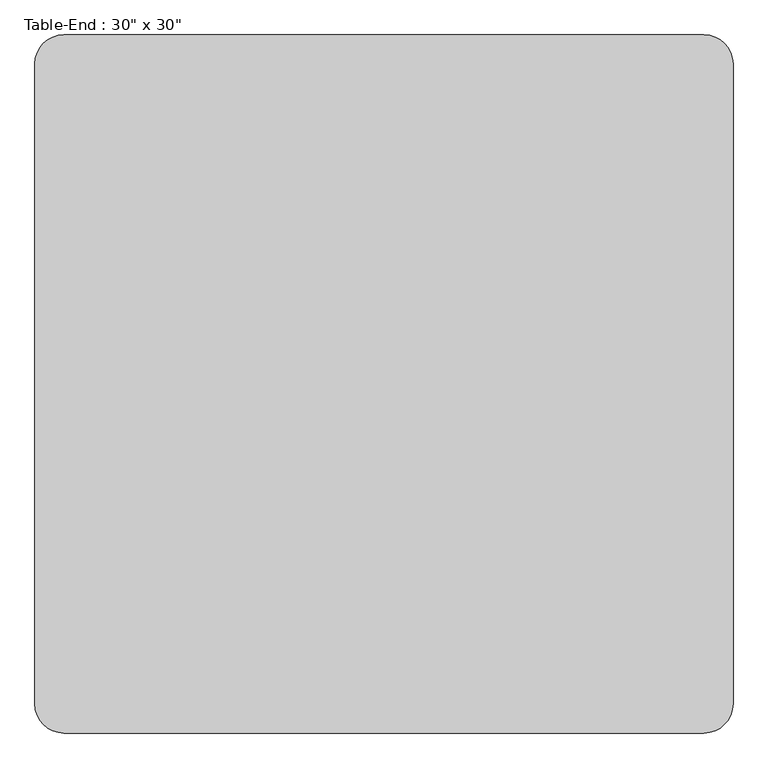
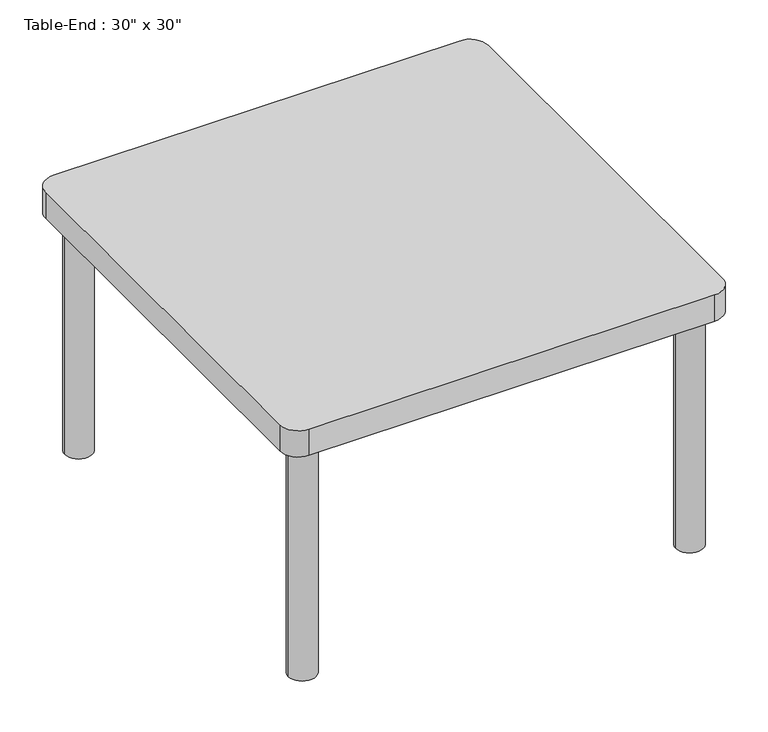
"""IFC4 building model written with IfcOpenShell, lengths in millimetres: furniture geometry."""

from ifc_helpers import new_model, si_unit, point, frame, frame_2d, origin, origin_with_axes, place, context, project, spatial, polyline, circle_curve, trimmed, segment, composite_curve, outline, extrude, source, transform, mapped, element, save


def furniture_e4e19c7b(model_context):
    return source(origin(), model_context, "Body", "SweptSolid", [
        extrude(outline(composite_curve([segment(polyline([(1172.1336303, -457.2), (54.5336303, -457.2)]), True, "CONTINUOUS"), segment(trimmed(circle_curve(frame_2d((54.5336303, -406.4)), 50.8), [point((54.5336303, -457.2))], [point((3.7336303, -406.4))], False, "CARTESIAN"), True, "CONTINUOUS"), segment(polyline([(3.7336303, -406.4), (3.7336303, 711.2)]), True, "CONTINUOUS"), segment(trimmed(circle_curve(frame_2d((54.5336303, 711.2)), 50.8), [point((3.7336303, 711.2))], [point((54.5336303, 762.0))], False, "CARTESIAN"), True, "CONTINUOUS"), segment(polyline([(54.5336303, 762.0), (1172.1336303, 762.0)]), True, "CONTINUOUS"), segment(trimmed(circle_curve(frame_2d((1172.1336303, 711.2)), 50.8), [point((1172.1336303, 762.0))], [point((1222.9336303, 711.2))], False, "CARTESIAN"), True, "CONTINUOUS"), segment(polyline([(1222.9336303, 711.2), (1222.9336303, -406.4)]), True, "CONTINUOUS"), segment(trimmed(circle_curve(frame_2d((1172.1336303, -406.4)), 50.8), [point((1222.9336303, -406.4))], [point((1172.1336303, -457.2))], False, "CARTESIAN"), True, "CONTINUOUS")], self_intersect=False)), frame((0.0, 0.0, 685.8), z_axis=(0.0, 0.0, 1.0), x_axis=(1.0, 0.0, 0.0)), (0.0, 0.0, 1.0), 76.2),
        extrude(outline(composite_curve([segment(trimmed(circle_curve(frame_2d((79.9336303, 685.8)), 38.1), [point((41.8336303, 685.8))], [point((118.0336303, 685.8))], False, "CARTESIAN"), True, "CONTINUOUS"), segment(trimmed(circle_curve(frame_2d((79.9336303, 685.8)), 38.1), [point((118.0336303, 685.8))], [point((41.8336303, 685.8))], False, "CARTESIAN"), True, "CONTINUOUS")], self_intersect=False)), origin_with_axes(), (0.0, 0.0, 1.0), 685.8),
        extrude(outline(composite_curve([segment(trimmed(circle_curve(frame_2d((79.9336303, -381.0)), 38.1), [point((41.8336303, -381.0))], [point((118.0336303, -381.0))], False, "CARTESIAN"), True, "CONTINUOUS"), segment(trimmed(circle_curve(frame_2d((79.9336303, -381.0)), 38.1), [point((118.0336303, -381.0))], [point((41.8336303, -381.0))], False, "CARTESIAN"), True, "CONTINUOUS")], self_intersect=False)), origin_with_axes(), (0.0, 0.0, 1.0), 685.8),
        extrude(outline(composite_curve([segment(trimmed(circle_curve(frame_2d((1146.7336303, -381.0)), 38.1), [point((1108.6336303, -381.0))], [point((1184.8336303, -381.0))], False, "CARTESIAN"), True, "CONTINUOUS"), segment(trimmed(circle_curve(frame_2d((1146.7336303, -381.0)), 38.1), [point((1184.8336303, -381.0))], [point((1108.6336303, -381.0))], False, "CARTESIAN"), True, "CONTINUOUS")], self_intersect=False)), origin_with_axes(), (0.0, 0.0, 1.0), 685.8),
        extrude(outline(composite_curve([segment(trimmed(circle_curve(frame_2d((1146.7336303, 685.8)), 38.1), [point((1108.6336303, 685.8))], [point((1184.8336303, 685.8))], False, "CARTESIAN"), True, "CONTINUOUS"), segment(trimmed(circle_curve(frame_2d((1146.7336303, 685.8)), 38.1), [point((1184.8336303, 685.8))], [point((1108.6336303, 685.8))], False, "CARTESIAN"), True, "CONTINUOUS")], self_intersect=False)), origin_with_axes(), (0.0, 0.0, 1.0), 685.8),
    ])


if __name__ == "__main__":
    model = new_model("IFC4")
    model_context = context("Model", 3, world=origin())
    ifc_project = project(units=[si_unit("LENGTHUNIT", "METRE", prefix="MILLI")], contexts=[model_context])
    site = spatial("IfcSite", under=ifc_project)
    building = spatial("IfcBuilding", under=site)
    placement = place(None, origin())
    furniture_shape = furniture_e4e19c7b(model_context)
    element("IfcFurniture", 1, ObjectType="Table-End : 30\" x 30\"", at=placement, inside=building, context=model_context, shape_type="MappedRepresentation", body=[
        mapped(furniture_shape, transform((0.0, 0.0, 0.0), x_axis=(1.0, 0.0, 0.0), y_axis=(0.0, 1.0, 0.0), z_axis=(0.0, 0.0, 1.0))),
    ])
    save(model, "model.ifc")

# Revit data of these elements
# Type "Table-End : 30\" x 30\""
#   Assembly Code = "E2020200"
#   Height = 2' - 6"
#   Length = 4' - 0"
#   Width = 4' - 0"
#   Base Material = Birch
#   Top Material = Laminate, Ivory, Matte
#   Default Elevation = 0
# Element 1 (IfcFurniture, "Table-End : 30\" x 30\"")
#   Materials on its faces: "Laminate, Ivory, Matte", "Birch"
# Materials
#   "Birch": class "Wood", colour RGB 224 178 126, transparency 0, Description = "Betula Alleghaniensis", Cost = 0
#   "Laminate, Ivory, Matte": class "Plastic", colour RGB 247 247 239, transparency 0, Description = "Plastic Laminate - Ivory, Matte", Cost = 0
